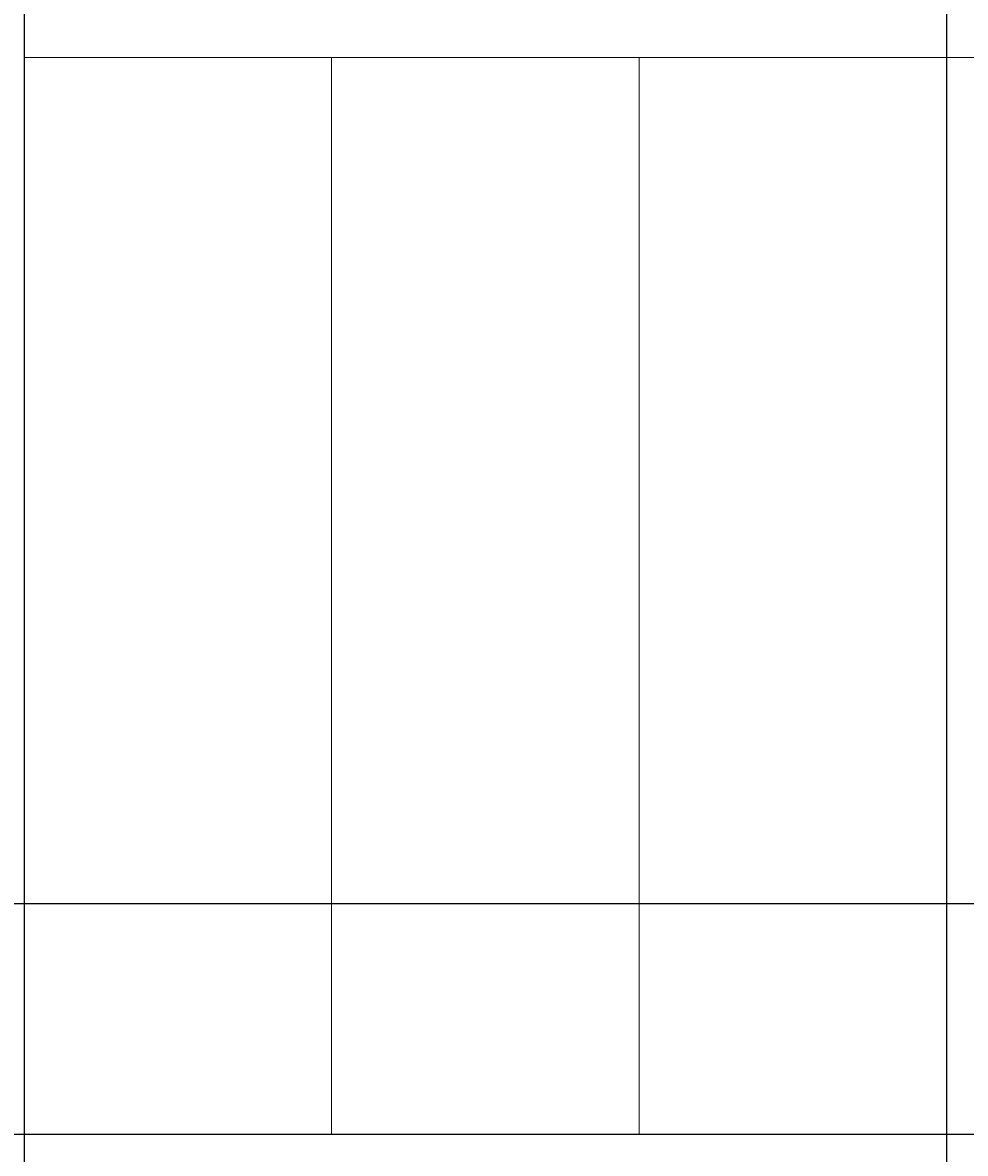
# Model space of a CAD drawing. Units: feet. Extents: x 1654 to 2985, y 1348 to 2230.
# Tile 19 of 53: x 2130 to 2167, y 1565 to 1609. Entities that reach past the tile are written whole.
import ezdxf

# ---------------------------------------------------------------- set-up
doc = ezdxf.new("R2010")
doc.units = ezdxf.units.FT
for name, color, linetype, lineweight in [('A-ANNO-DIMS', 2, 'Continuous', 18), ('A-FLOR', 7, 'Continuous', 25), ('A-FLOR-STRS', 7, 'Continuous', 18)]:
    doc.layers.add(name, color=color, linetype=linetype, lineweight=lineweight)
doc.styles.get("Standard").update_dxf_attribs({"font": 'arial.ttf'})
doc.dimstyles.get("Standard").update_dxf_attribs({"dimtxt": 0.18, "dimasz": 0.18, "dimexe": 0.18, "dimexo": 0.0625, "dimgap": 0.09, "dimtad": 0, "dimtih": 1, "dimtoh": 1, "dimdec": 4, "dimzin": 0, "dimdsep": 46, "dimtxsty": 'Standard', "dimcen": 0.09, "dimadec": 0, "dimazin": 0, "dimtfac": 1, "dimtdec": 4, "dimtofl": 0, "dimtmove": 0, "dimatfit": 3, "dimfxl": 1, "dimtolj": 1, "dimtzin": 0, "dimarcsym": 0})

# ---------------------------------------------------------------- blocks, each defined once
blk = doc.blocks.new('STAIR-RETURN')
for p, q in [((36, 186), (36, 0)), ((0, 42), (72, 42)), ((0, 42), (0, 0)), ((12, 42), (12, 0)), ((24, 42), (24, 0))]:
    blk.add_line(p, q)
blk = doc.blocks.new('*D73')
at = {"layer": 'A-ANNO-DIMS', "color": 0, "lineweight": -2, "transparency": 16777216}
for p, q in [((2130.092, 1565.192), (2130.092, 1537.175)), ((2202.092, 1565.192), (2202.092, 1537.175)), ((2130.272, 1537.355), (2165.565, 1537.355)), ((2201.912, 1537.355), (2166.62, 1537.355))]:
    blk.add_line(p, q, dxfattribs=at)
at = {"layer": 'A-ANNO-DIMS', "color": 0, "transparency": 16777216}
for points in [[(2130.272, 1537.385), (2130.272, 1537.325), (2130.092, 1537.355)], [(2201.912, 1537.385), (2201.912, 1537.325), (2202.092, 1537.355)]]:
    blk.add_solid(points, dxfattribs=at)
at = {"layer": 'Defpoints', "color": 0, "transparency": 16777216}
for p in [(2130.092, 1565.255), (2202.092, 1565.255), (2202.092, 1537.355)]:
    blk.add_point(p, dxfattribs=at)
at = {"layer": 'A-ANNO-DIMS', "color": 0, "transparency": 16777216, "insert": (2166.092, 1537.355), "char_height": 0.18, "attachment_point": 5}
blk.add_mtext('\\A1;72 TYP.', dxfattribs=at)
blk = doc.blocks.new('*D80')
at = {"layer": 'A-ANNO-DIMS', "color": 0, "lineweight": -2, "transparency": 16777216}
for p, q in [((2070.092, 2039.192), (2070.092, 1534.075)), ((2202.092, 2039.192), (2202.092, 1534.075)), ((2070.272, 1534.255), (2135.813, 1534.255)), ((2201.912, 1534.255), (2136.372, 1534.255))]:
    blk.add_line(p, q, dxfattribs=at)
at = {"layer": 'A-ANNO-DIMS', "color": 0, "transparency": 16777216}
for points in [[(2070.272, 1534.285), (2070.272, 1534.225), (2070.092, 1534.255)], [(2201.912, 1534.285), (2201.912, 1534.225), (2202.092, 1534.255)]]:
    blk.add_solid(points, dxfattribs=at)
at = {"layer": 'Defpoints', "color": 0, "transparency": 16777216}
for p in [(2070.092, 2039.255), (2202.092, 2039.255), (2202.092, 1534.255)]:
    blk.add_point(p, dxfattribs=at)
at = {"layer": 'A-ANNO-DIMS', "color": 0, "transparency": 16777216, "insert": (2136.092, 1534.255), "char_height": 0.18, "attachment_point": 5}
blk.add_mtext('\\A1;132', dxfattribs=at)
blk = doc.blocks.new('*D90')
at = {"layer": 'A-ANNO-DIMS', "color": 0, "lineweight": -2, "transparency": 16777216}
for p, q in [((1852.155, 1641.187), (2242.272, 1641.187)), ((2242.092, 1641.007), (2242.092, 1607.903)), ((2242.092, 1574.435), (2242.092, 1607.539)), ((1852.155, 1574.255), (2242.272, 1574.255))]:
    blk.add_line(p, q, dxfattribs=at)
at = {"layer": 'A-ANNO-DIMS', "color": 0, "transparency": 16777216}
for points in [[(2242.062, 1641.007), (2242.122, 1641.007), (2242.092, 1641.187)], [(2242.062, 1574.435), (2242.122, 1574.435), (2242.092, 1574.255)]]:
    blk.add_solid(points, dxfattribs=at)
at = {"layer": 'Defpoints', "color": 0, "transparency": 16777216}
for p in [(1852.092, 1641.187), (2242.092, 1641.187), (1852.092, 1574.255)]:
    blk.add_point(p, dxfattribs=at)
at = {"layer": 'A-ANNO-DIMS', "color": 0, "transparency": 16777216, "insert": (2242.092, 1607.721), "char_height": 0.18, "attachment_point": 5}
blk.add_mtext('\\A1;66.93', dxfattribs=at)
blk = doc.blocks.new('*D99')
at = {"layer": 'A-ANNO-DIMS', "color": 0, "lineweight": -2, "transparency": 16777216}
for p, q in [((2166.092, 1746.692), (2166.092, 1534.075)), ((2130.092, 1742.192), (2130.092, 1534.075)), ((2130.272, 1534.255), (2147.874, 1534.255)), ((2165.912, 1534.255), (2148.311, 1534.255))]:
    blk.add_line(p, q, dxfattribs=at)
at = {"layer": 'A-ANNO-DIMS', "color": 0, "transparency": 16777216}
for points in [[(2130.272, 1534.285), (2130.272, 1534.225), (2130.092, 1534.255)], [(2165.912, 1534.285), (2165.912, 1534.225), (2166.092, 1534.255)]]:
    blk.add_solid(points, dxfattribs=at)
at = {"layer": 'Defpoints', "color": 0, "transparency": 16777216}
for p in [(2166.092, 1746.755), (2130.092, 1742.255), (2166.092, 1534.255)]:
    blk.add_point(p, dxfattribs=at)
at = {"layer": 'A-ANNO-DIMS', "color": 0, "transparency": 16777216, "insert": (2148.092, 1534.255), "char_height": 0.18, "attachment_point": 5}
blk.add_mtext('\\A1;36', dxfattribs=at)
blk = doc.blocks.new('*D103')
at = {"layer": 'A-ANNO-DIMS', "color": 0, "lineweight": -2, "transparency": 16777216}
for p, q in [((2070.092, 1661.192), (2070.092, 1534.075)), ((2130.092, 1565.192), (2130.092, 1534.075)), ((2070.272, 1534.255), (2099.873, 1534.255)), ((2129.912, 1534.255), (2100.312, 1534.255))]:
    blk.add_line(p, q, dxfattribs=at)
at = {"layer": 'A-ANNO-DIMS', "color": 0, "transparency": 16777216}
for points in [[(2070.272, 1534.285), (2070.272, 1534.225), (2070.092, 1534.255)], [(2129.912, 1534.285), (2129.912, 1534.225), (2130.092, 1534.255)]]:
    blk.add_solid(points, dxfattribs=at)
at = {"layer": 'Defpoints', "color": 0, "transparency": 16777216}
for p in [(2070.092, 1661.255), (2130.092, 1565.255), (2130.092, 1534.255)]:
    blk.add_point(p, dxfattribs=at)
at = {"layer": 'A-ANNO-DIMS', "color": 0, "transparency": 16777216, "insert": (2100.092, 1534.255), "char_height": 0.18, "attachment_point": 5}
blk.add_mtext('\\A1;60', dxfattribs=at)

msp = doc.modelspace()

# ---------------------------------------------------------------- linework, layer by layer
at = {"layer": 'A-FLOR'}
msp.add_line((2008.0924, 1565.2549), (2211.0924, 1565.2549), dxfattribs=at)

# ---------------------------------------------------------------- block references
at = {"layer": 'A-FLOR-STRS'}
msp.add_blockref('STAIR-RETURN', (2130.092, 1565.255), dxfattribs=at)

# ---------------------------------------------------------------- dimensions: what is measured, and where the dimension line sits
at = {"layer": 'A-ANNO-DIMS'}
for base, p1, p2, picture, middle in [((2202.0924, 1534.2549), (2070.0924, 2039.2549), (2202.0924, 2039.2549), '*D80', (2136.0924, 1534.2549)), ((2166.0924, 1534.2549), (2130.0924, 1742.2549), (2166.0924, 1746.7549), '*D99', (2148.0924, 1534.2549)), ((2130.0924, 1534.2549), (2070.0924, 1661.2549), (2130.0924, 1565.2549), '*D103', (2100.0924, 1534.2549))]:
    dim = msp.add_linear_dim(base=base, p1=p1, p2=p2, dimstyle='Standard', override={"dimdec": 0, "dimlfac": 1, "dimrnd": 0, "dimzin": 0, "dimdsep": 46, "dimlunit": 2}, dxfattribs=at)
    dim.commit()
    dim.dimension.update_dxf_attribs({"geometry": picture, "text_midpoint": middle})
dim = msp.add_linear_dim(base=(2242.0924, 1641.187), p1=(1852.0924, 1574.2549), p2=(1852.0924, 1641.187), angle=90, dimstyle='Standard', override={"dimdec": 2, "dimlfac": 1, "dimrnd": 0, "dimzin": 0, "dimdsep": 46, "dimlunit": 2}, dxfattribs=at)
dim.commit()
dim.dimension.update_dxf_attribs({"geometry": '*D90', "text_midpoint": (2242.0924, 1607.721)})
dim = msp.add_linear_dim(base=(2202.0924, 1537.3549), p1=(2130.0924, 1565.2549), p2=(2202.0924, 1565.2549), text='<> TYP.', dimstyle='Standard', override={"dimdec": 0, "dimlfac": 1, "dimrnd": 0, "dimzin": 0, "dimdsep": 46, "dimlunit": 2}, dxfattribs=at)
dim.commit()
dim.dimension.update_dxf_attribs({"geometry": '*D73', "text_midpoint": (2166.0924, 1537.3549)})

doc.saveas('drawing.dxf')
